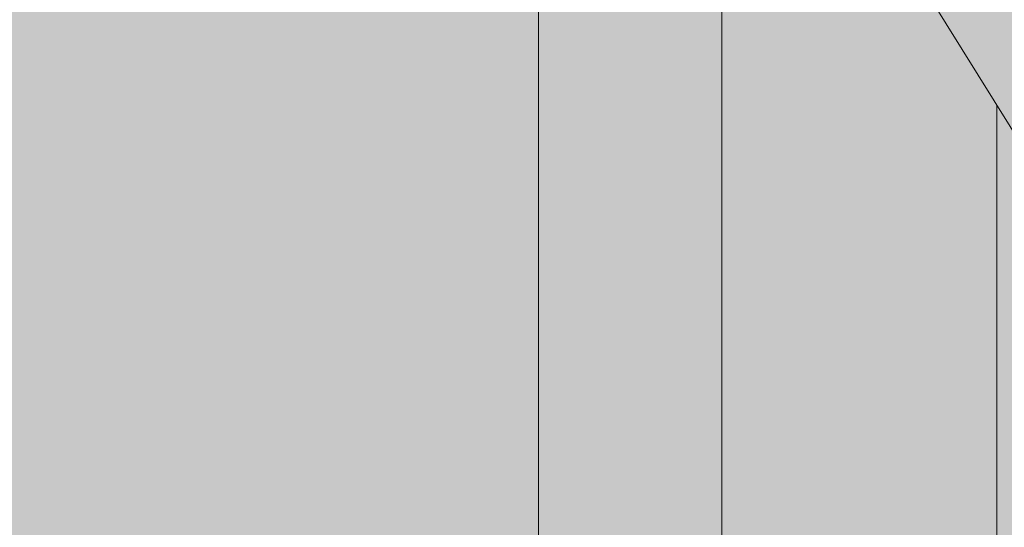
# Model space of a CAD drawing. Units: millimetres. Extents: x 11032 to 26788, y 3406 to 24505.
# Tile 46 of 78: x 15518 to 15786, y 16039 to 16177. Entities that reach past the tile are written whole.
import ezdxf

# ---------------------------------------------------------------- set-up
doc = ezdxf.new("R2010")
doc.units = ezdxf.units.MM
doc.header["$MEASUREMENT"] = 0
for name, color, linetype, lineweight in [('A-ANNO-DIMS', 2, 'Continuous', 18), ('A-GLAZ', 250, 'Continuous', 20), ('A-ROOF', 7, 'Continuous', 30), ('A-WALL', 7, 'Continuous', 35), ('E-LITE', 7, 'Continuous', 18), ('E-LITE-PATT', 7, 'Continuous', 13)]:
    doc.layers.add(name, color=color, linetype=linetype, lineweight=lineweight)
for name, color, linetype, lineweight, true_color in [('A-GLAZ-FRAM-PATT', 250, 'Continuous', 13, 0x262627), ('A-ROOF-PATT', 9, 'Continuous', 13, 0xc7c8ca), ('A-WALL-INTR-PATT', 251, 'Continuous', 13, 0x6c6b6a)]:
    doc.layers.add(name, color=color, linetype=linetype, lineweight=lineweight, true_color=true_color)
doc.styles.get("Standard").update_dxf_attribs({"font": 'arial.ttf'})
doc.dimstyles.get("Standard").update_dxf_attribs({"dimtxt": 150, "dimasz": 100, "dimexe": 10, "dimexo": 5, "dimgap": 5, "dimtad": 0, "dimtih": 1, "dimtoh": 1, "dimdec": 0, "dimzin": 0, "dimdsep": 46, "dimtxsty": 'Standard', "dimcen": 0.09, "dimadec": 0, "dimazin": 0, "dimtfac": 1, "dimtdec": 0, "dimtofl": 0, "dimtmove": 0, "dimatfit": 3, "dimfxl": 1, "dimtolj": 1, "dimtzin": 0, "dimarcsym": 0})

# ---------------------------------------------------------------- blocks, each defined once
blk = doc.blocks.new('*D36')
at = {"layer": 'A-ANNO-DIMS', "color": 0, "lineweight": -2, "transparency": 16777216}
for p, q in [((12301.26, 17115.89), (12301.26, 24416.86)), ((25397.4, 4466.4), (25397.4, 24416.86)), ((12401.26, 24406.86), (18569.2, 24406.86)), ((25297.4, 24406.86), (19129.47, 24406.86))]:
    blk.add_line(p, q, dxfattribs=at)
at = {"layer": 'A-ANNO-DIMS', "color": 0, "transparency": 16777216}
for points in [[(12401.26, 24423.52), (12401.26, 24390.19), (12301.26, 24406.86)], [(25297.4, 24423.52), (25297.4, 24390.19), (25397.4, 24406.86)]]:
    blk.add_solid(points, dxfattribs=at)
at = {"layer": 'Defpoints', "color": 0, "transparency": 16777216}
for p in [(25397.4, 24406.86), (12301.26, 17110.89), (25397.4, 4461.4)]:
    blk.add_point(p, dxfattribs=at)
at = {"layer": 'A-ANNO-DIMS', "color": 0, "transparency": 16777216, "insert": (18849.33, 24406.86), "char_height": 150, "attachment_point": 5}
blk.add_mtext('\\A1;13096', dxfattribs=at)
blk = doc.blocks.new('*D37')
at = {"layer": 'A-ANNO-DIMS', "color": 0, "lineweight": -2, "transparency": 16777216}
for p, q in [((18087.74, 23450.36), (11334.76, 23450.36)), ((11344.76, 23350.36), (11344.76, 14037.46)), ((11344.76, 4561.4), (11344.76, 13874.29)), ((12927.66, 4461.4), (11334.76, 4461.4))]:
    blk.add_line(p, q, dxfattribs=at)
at = {"layer": 'A-ANNO-DIMS', "color": 0, "transparency": 16777216}
for points in [[(11328.1, 23350.36), (11361.43, 23350.36), (11344.76, 23450.36)], [(11328.1, 4561.4), (11361.43, 4561.4), (11344.76, 4461.4)]]:
    blk.add_solid(points, dxfattribs=at)
at = {"layer": 'Defpoints', "color": 0, "transparency": 16777216}
for p in [(11344.76, 23450.36), (18092.74, 23450.36), (12932.66, 4461.4)]:
    blk.add_point(p, dxfattribs=at)
at = {"layer": 'A-ANNO-DIMS', "color": 0, "transparency": 16777216, "insert": (11344.76, 13955.88), "char_height": 150, "attachment_point": 5}
blk.add_mtext('\\A1;18989', dxfattribs=at)
blk = doc.blocks.new('*D57')
at = {"layer": 'A-ANNO-DIMS', "color": 0, "lineweight": -2, "transparency": 16777216}
for p, q in [((14994.7, 7266.4), (14994.7, 24416.86)), ((20894.7, 7266.4), (20894.7, 24416.86)), ((15094.7, 24406.86), (17715.98, 24406.86)), ((20794.7, 24406.86), (18173.42, 24406.86))]:
    blk.add_line(p, q, dxfattribs=at)
at = {"layer": 'A-ANNO-DIMS', "color": 0, "transparency": 16777216}
for points in [[(15094.7, 24423.52), (15094.7, 24390.19), (14994.7, 24406.86)], [(20794.7, 24423.52), (20794.7, 24390.19), (20894.7, 24406.86)]]:
    blk.add_solid(points, dxfattribs=at)
at = {"layer": 'Defpoints', "color": 0, "transparency": 16777216}
for p in [(20894.7, 24406.86), (14994.7, 7261.4), (20894.7, 7261.4)]:
    blk.add_point(p, dxfattribs=at)
at = {"layer": 'A-ANNO-DIMS', "color": 0, "transparency": 16777216, "insert": (17944.7, 24406.86), "char_height": 150, "attachment_point": 5}
blk.add_mtext('\\A1;5900', dxfattribs=at)
blk = doc.blocks.new('*D60')
at = {"layer": 'A-ANNO-DIMS', "color": 0, "lineweight": -2, "transparency": 16777216}
for p, q in [((14994.7, 7266.4), (14994.7, 24416.86)), ((16344.7, 7266.4), (16344.7, 24416.86)), ((15094.7, 24406.86), (15448.04, 24406.86)), ((16244.7, 24406.86), (15891.36, 24406.86))]:
    blk.add_line(p, q, dxfattribs=at)
at = {"layer": 'A-ANNO-DIMS', "color": 0, "transparency": 16777216}
for points in [[(15094.7, 24423.52), (15094.7, 24390.19), (14994.7, 24406.86)], [(16244.7, 24423.52), (16244.7, 24390.19), (16344.7, 24406.86)]]:
    blk.add_solid(points, dxfattribs=at)
at = {"layer": 'Defpoints', "color": 0, "transparency": 16777216}
for p in [(16344.7, 24406.86), (14994.7, 7261.4), (16344.7, 7261.4)]:
    blk.add_point(p, dxfattribs=at)
at = {"layer": 'A-ANNO-DIMS', "color": 0, "transparency": 16777216, "insert": (15669.7, 24406.86), "char_height": 150, "attachment_point": 5}
blk.add_mtext('\\A1;1350', dxfattribs=at)

msp = doc.modelspace()

# ---------------------------------------------------------------- hatches: boundary and pattern name
at = {"layer": 'A-GLAZ-FRAM-PATT'}
h = msp.add_hatch(color=256, dxfattribs=at)
edge = h.paths.add_edge_path()
edge.add_line((15284.393, 17051.32), (15084.393, 17001.32))
edge.add_line((15084.393, 17001.32), (15084.393, 15951.32))
edge.add_spline(control_points=[(15084.393, 15951.32), (15157.266, 15924.219), (15224.458, 15897.808), (15284.393, 15870.289)], knot_values=[511.9490104, 511.9490104, 511.9490104, 511.9490104, 697.3715979, 697.3715979, 697.3715979, 697.3715979], degree=3, periodic=0)
edge.add_line((15284.393, 15870.289), (15284.393, 17051.32))
edge = h.paths.add_edge_path()
edge.add_line((15659.393, 16354.387), (15459.393, 16675.629))
edge.add_line((15459.393, 16675.629), (15459.393, 15771.505))
edge.add_spline(control_points=[(15459.393, 15771.505), (15501.891, 15741.568), (15571.096, 15682.692), (15632.72, 15612.509), (15659.393, 15578.299)], knot_values=[905.064582, 905.064582, 905.064582, 905.064582, 1079.4682707, 1223.1584353, 1223.1584353, 1223.1584353, 1223.1584353], degree=3, periodic=0)
edge.add_line((15659.393, 15578.299), (15659.393, 16354.387))
h.paths.add_polyline_path([(15284.393, 17051.32), (15284.393, 16956.717), (15784.393, 16153.61), (15784.393, 16248.213)])
h = msp.add_hatch(color=256, dxfattribs=at)
edge = h.paths.add_edge_path()
edge.add_spline(control_points=[(15409.393, 16728.446), (15384.197, 16718.122), (15359.177, 16707.259), (15334.393, 16695.842)], knot_values=[2052.6714029, 2052.6714029, 2052.6714029, 2052.6714029, 2131.0201637, 2131.0201637, 2131.0201637, 2131.0201637], degree=3, periodic=0)
edge.add_line((15334.393, 16695.842), (15334.393, 15846.165))
edge.add_spline(control_points=[(15334.393, 15846.165), (15360.99, 15832.635), (15385.89, 15818.741), (15409.393, 15804.345)], knot_values=[750.8383504, 750.8383504, 750.8383504, 750.8383504, 839.4758736, 839.4758736, 839.4758736, 839.4758736], degree=3, periodic=0)
edge.add_line((15409.393, 15804.345), (15409.393, 16728.446))
edge = h.paths.add_edge_path()
edge.add_line((15784.393, 16153.61), (15709.393, 16274.076))
edge.add_line((15709.393, 16274.076), (15709.393, 15509.31))
edge.add_spline(control_points=[(15709.393, 15509.31), (15712.398, 15504.862), (15738.373, 15465.922), (15763.422, 15424.165), (15784.393, 15385.996)], knot_values=[1315.3424293, 1315.3424293, 1315.3424293, 1315.3424293, 1332.3824154, 1463.2850479, 1463.2850479, 1463.2850479, 1463.2850479], degree=3, periodic=0)
edge.add_line((15784.393, 15385.996), (15784.393, 16153.61))
h = msp.add_hatch(color=256, dxfattribs=at)
edge = h.paths.add_edge_path()
edge.add_line((15784.393, 16248.213), (15784.393, 16153.61))
edge.add_line((15784.393, 16153.61), (16560.042, 14907.752))
edge.add_spline(control_points=[(16560.042, 14907.752), (16569.192, 14907.664), (16578.343, 14907.575), (16587.493, 14907.486), (16598.103, 14907.383), (16608.713, 14907.281), (16619.296, 14907.181)], knot_values=[1012.2878735, 1012.2878735, 1012.2878735, 1012.2878735, 1027.155312, 1027.155312, 1027.155312, 1044.3939449, 1044.3939449, 1044.3939449, 1044.3939449], degree=3, periodic=0)
edge.add_line((16619.296, 14907.181), (15784.393, 16248.213))
at = {"layer": 'A-ROOF-PATT'}
h = msp.add_hatch(color=256, dxfattribs=at)
edge = h.paths.add_edge_path()
edge.add_spline(control_points=[(17532.827, 17324.837), (17391.335, 17349.016), (16840.872, 17494.912), (16080.055, 18069.544), (14738.803, 18299.641), (13382.429, 18838.336), (12580.532, 17870.207), (12430.422, 17563.822)], knot_values=[2977.6027945, 2977.6027945, 2977.6027945, 2977.6027945, 3438.1840601, 4811.6463022, 5622.8675483, 7588.0288188, 8560.6685791, 8560.6685791, 8560.6685791, 8560.6685791], degree=3, periodic=0)
edge.add_spline(control_points=[(12430.422, 17563.822), (12437.904, 17573.36), (12445.386, 17582.899), (12452.869, 17592.437), (12452.869, 17592.438), (12452.869, 17592.438), (12452.869, 17592.438)], knot_values=[1408.564138, 1408.564138, 1408.564138, 1408.564138, 1444.85989, 1444.85989, 1444.85989, 1444.8601183, 1444.8601183, 1444.8601183, 1444.8601183], degree=3, periodic=0)
edge.add_spline(control_points=[(12452.869, 17592.438), (12555.432, 17723.185), (12736.557, 17929.686), (13044.86, 18114.643), (13219.943, 18189.644), (13299.92, 18220.646)], knot_values=[339.318246, 339.318246, 339.318246, 339.318246, 836.8349967, 1151.2512933, 1408.564138, 1408.564138, 1408.564138, 1408.564138], degree=3, periodic=0)
edge.add_spline(control_points=[(13299.92, 18220.646), (13299.998, 18220.689), (13300.077, 18220.732), (13319.738, 18231.488), (13339.24, 18241.402), (13388.645, 18264.703), (13418.466, 18277.069), (13478.019, 18298.648), (13507.751, 18307.861), (13544.561, 18317.488), (13551.584, 18319.245), (13558.612, 18320.924)], knot_values=[3783.8950972, 3783.8950972, 3783.8950972, 3783.8950972, 3784.1737101, 3784.1737101, 3853.4666747, 3853.4666747, 3960.2401917, 3960.2401917, 4067.0137087, 4067.0137087, 4092.1744649, 4092.1744649, 4092.1744649, 4092.1744649], degree=3, periodic=0)
edge.add_spline(control_points=[(13558.612, 18320.924), (13581.407, 18326.373), (13604.25, 18331.007), (13657.184, 18339.957), (13687.338, 18343.732), (13748.098, 18348.892), (13778.704, 18350.276), (13840.46, 18350.833), (13871.609, 18350.005), (13934.496, 18346.313), (13966.232, 18343.449), (14030.297, 18335.871), (14062.625, 18331.158), (14127.853, 18320.088), (14160.753, 18313.73), (14241.357, 18296.556), (14289.343, 18284.997), (14386.31, 18259.688), (14435.291, 18245.941), (14534.161, 18217.034), (14584.049, 18201.875), (14684.682, 18170.964), (14735.427, 18155.212), (14837.763, 18123.971), (14889.354, 18108.482), (14954.971, 18089.677), (14968.586, 18085.823), (14992.391, 18079.184), (15002.566, 18076.376), (15021.739, 18071.153), (15030.731, 18068.729), (15047.707, 18064.21), (15055.694, 18062.106), (15079.815, 18055.825), (15095.905, 18051.728), (15143.966, 18039.717), (15175.729, 18032.084), (15254.84, 18013.501), (15301.798, 18002.866), (15394.186, 17981.845), (15439.615, 17971.459), (15528.833, 17950.135), (15572.62, 17939.197), (15658.477, 17916.021), (15700.546, 17903.785), (15753.633, 17886.734), (15765.446, 17882.835), (15786.574, 17875.653), (15795.915, 17872.404), (15810.108, 17867.349), (15814.99, 17865.588), (15824.736, 17862.029), (15829.611, 17860.226), (15844.241, 17854.75), (15854.002, 17851.008), (15883.312, 17839.521), (15902.885, 17831.512), (15966.355, 17804.548), (16010.39, 17784.302), (16098.838, 17741.267), (16143.25, 17718.478), (16232.497, 17671.098), (16277.332, 17646.507), (16367.515, 17596.295), (16412.862, 17570.676), (16504.202, 17519.209), (16550.194, 17493.362), (16643.009, 17442.263), (16689.831, 17417.011), (16756.517, 17382.472), (16775.937, 17372.58), (16795.455, 17362.84)], knot_values=[4092.1744649, 4092.1744649, 4092.1744649, 4092.1744649, 4173.7872258, 4173.7872258, 4280.5607428, 4280.5607428, 4387.3342598, 4387.3342598, 4494.1077768, 4494.1077768, 4600.8812939, 4600.8812939, 4707.6548109, 4707.6548109, 4814.4283279, 4814.4283279, 4967.1262405, 4967.1262405, 5119.8241531, 5119.8241531, 5272.5220657, 5272.5220657, 5425.2199783, 5425.2199783, 5577.9178908, 5577.9178908, 5617.7853319, 5617.7853319, 5647.4648479, 5647.4648479, 5673.611025, 5673.611025, 5696.747607, 5696.747607, 5743.6818903, 5743.6818903, 5837.5504571, 5837.5504571, 5979.7261046, 5979.7261046, 6121.9017521, 6121.9017521, 6264.0773996, 6264.0773996, 6406.2530471, 6406.2530471, 6447.2585849, 6447.2585849, 6480.0420882, 6480.0420882, 6497.3077062, 6497.3077062, 6514.5733242, 6514.5733242, 6549.1045602, 6549.1045602, 6618.1670322, 6618.1670322, 6772.6610171, 6772.6610171, 6927.155002, 6927.155002, 7081.6489869, 7081.6489869, 7236.1429718, 7236.1429718, 7390.6369567, 7390.6369567, 7545.1309416, 7545.1309416, 7608.1992868, 7608.1992868, 7608.1992868, 7608.1992868], degree=3, periodic=0)
edge.add_spline(control_points=[(16795.455, 17362.84), (16814.335, 17349.456), (16832.897, 17336.263), (16873.225, 17307.197), (16894.778, 17291.386), (16936.221, 17259.941), (16956.11, 17244.308), (16993.863, 17213.094), (17011.726, 17197.514), (17041.993, 17169.265), (17054.791, 17156.601), (17078.762, 17131.225), (17089.933, 17118.516), (17110.618, 17092.991), (17120.131, 17080.178), (17130.17, 17065.264), (17131.487, 17063.277), (17133.77, 17059.776), (17134.746, 17058.261), (17136.69, 17055.205), (17137.657, 17053.668), (17140.539, 17049.025), (17142.438, 17045.89), (17148.068, 17036.367), (17151.732, 17029.859), (17163.03, 17008.788), (17170.335, 16993.646), (17184.087, 16961.978), (17190.534, 16945.453), (17202.562, 16911.165), (17208.142, 16893.402), (17218.448, 16856.821), (17223.173, 16838.003), (17231.801, 16799.51), (17235.705, 16779.837), (17241.533, 16746.739), (17243.676, 16733.5), (17247.718, 16706.37), (17249.608, 16692.472), (17252.066, 16672.69), (17252.761, 16666.875), (17254.1, 16655.226), (17254.744, 16649.4), (17256.596, 16631.917), (17257.727, 16620.254), (17260.823, 16585.238), (17262.489, 16561.858), (17266.551, 16488.654), (17267.658, 16438.661), (17267.349, 16375.228), (17267.193, 16362.07), (17266.95, 16348.891)], knot_values=[15.1130472, 15.1130472, 15.1130472, 15.1130472, 82.6995146, 82.6995146, 165.3990291, 165.3990291, 248.0985437, 248.0985437, 330.7980583, 330.7980583, 397.9419458, 397.9419458, 465.0858333, 465.0858333, 532.2297209, 532.2297209, 542.533741, 542.533741, 550.3568158, 550.3568158, 558.1798906, 558.1798906, 573.8260402, 573.8260402, 605.1183395, 605.1183395, 672.7640614, 672.7640614, 740.4097834, 740.4097834, 808.0555054, 808.0555054, 875.7012273, 875.7012273, 943.3469493, 943.3469493, 987.6613492, 987.6613492, 1033.4121612, 1033.4121612, 1052.3850876, 1052.3850876, 1071.358014, 1071.358014, 1109.3038668, 1109.3038668, 1185.1955724, 1185.1955724, 1346.4419026, 1346.4419026, 1388.5586631, 1388.5586631, 1388.5586631, 1388.5586631], degree=3, periodic=0)
edge.add_spline(control_points=[(17266.95, 16348.891), (17266.95, 16348.891), (17266.95, 16348.891), (17266.95, 16348.891), (17253.182, 15602.417), (17239.414, 14855.943), (17225.646, 14109.469)], knot_values=[1388.5586631, 1388.5586631, 1388.5586631, 1388.5586631, 1388.5589654, 1388.5589654, 1388.5589654, 3774.0767661, 3774.0767661, 3774.0767661, 3774.0767661], degree=3, periodic=0)
edge.add_spline(control_points=[(17225.646, 14109.469), (17226.198, 14109.827), (17226.748, 14110.185), (17242.065, 14120.191), (17255.956, 14130.116), (17274.422, 14144.286), (17279.609, 14148.386), (17284.686, 14152.511)], knot_values=[1926.3423968, 1926.3423968, 1926.3423968, 1926.3423968, 1927.316729, 1927.316729, 1953.5121761, 1953.5121761, 1964.0732348, 1964.0732348, 1964.0732348, 1964.0732348], degree=3, periodic=0)
edge.add_spline(control_points=[(17284.686, 14152.511), (17315.791, 14194.761), (17384.413, 14446.273), (17407.128, 14793.401), (17407.093, 15295.84), (17423.274, 15626.362), (17415.601, 15782.507)], knot_values=[0, 0, 0, 0, 163.2554674, 619.2296767, 1171.8624483, 1621.6355562, 1621.6355562, 1621.6355562, 1621.6355562], degree=3, periodic=0)
edge.add_spline(control_points=[(17415.601, 15782.507), (17438.21, 16077.57), (17410.495, 16533.484), (17390.893, 17030.649), (17301.082, 17169.349)], knot_values=[543.9784753, 543.9784753, 543.9784753, 543.9784753, 1452.9852767, 1960.0114926, 1960.0114926, 1960.0114926, 1960.0114926], degree=3, periodic=0)
edge.add_spline(control_points=[(17301.082, 17169.349), (17346.58, 17157.64), (17392.235, 17147.336), (17467.161, 17132.609), (17496.336, 17127.412), (17525.58, 17122.709)], knot_values=[8131.593939, 8131.593939, 8131.593939, 8131.593939, 8269.7349273, 8269.7349273, 8357.5016646, 8357.5016646, 8357.5016646, 8357.5016646], degree=3, periodic=0)
edge.add_line((17525.58, 17122.709), (17532.827, 17324.837))
edge = h.paths.add_edge_path(flags=17)
edge.add_spline(control_points=[(13340.537, 14602.706), (13316.172, 14726.456), (13323.666, 14932.342), (13637.836, 15081.117), (13863.248, 15171.051), (14002.1, 15224.503), (14058.539, 15244.876)], knot_values=[680.8931862, 680.8931862, 680.8931862, 680.8931862, 1033.4728289, 1337.4008326, 1604.7214264, 1784.2944722, 1784.2944722, 1784.2944722, 1784.2944722], degree=3, periodic=0)
edge.add_spline(control_points=[(14058.539, 15244.876), (14058.289, 15275.236), (14057.634, 15305.434), (14055.312, 15376.527), (14053.359, 15417.248), (14048.642, 15497.048), (14045.89, 15536.143), (14042.888, 15574.619)], knot_values=[6573.1065419, 6573.1065419, 6573.1065419, 6573.1065419, 6636.7330012, 6636.7330012, 6723.8890547, 6723.8890547, 6809.6328771, 6809.6328771, 6809.6328771, 6809.6328771], degree=3, periodic=0)
edge.add_spline(control_points=[(14042.888, 15574.619), (13546.54, 15403.221), (13074.735, 15143.241), (13277.36, 14695.339), (13340.537, 14602.706)], knot_values=[503.7925783, 503.7925783, 503.7925783, 503.7925783, 1728.1787606, 2051.34844, 2051.34844, 2051.34844, 2051.34844], degree=3, periodic=0)
h = msp.add_hatch(color=256, dxfattribs=at)
h.set_gradient(color1=(254, 234, 185), color2=(254, 204, 102), name='HEMISPHERICAL')
edge = h.paths.add_edge_path()
edge.add_line((15084.393, 17001.32), (15284.393, 17051.32))
edge.add_line((15284.393, 17051.32), (15470.537, 16752.334))
edge.add_spline(control_points=[(15470.537, 16752.334), (15683.311, 16831.508), (16106.827, 16912.335), (16625.609, 16876.997), (17083.498, 16357.78), (17257.801, 16180.113)], knot_values=[0, 0, 0, 0, 655.2936334, 1252.0157838, 1989.6162859, 1989.6162859, 1989.6162859, 1989.6162859], degree=3, periodic=0)
edge.add_spline(control_points=[(17257.801, 16180.113), (17260.851, 16236.372), (17263.9, 16292.632), (17266.95, 16348.891)], knot_values=[1132.9967717, 1132.9967717, 1132.9967717, 1132.9967717, 1198.0464225, 1198.0464225, 1198.0464225, 1198.0464225], degree=3, periodic=0)
edge.add_spline(control_points=[(17266.95, 16348.891), (17267.193, 16362.07), (17267.349, 16375.228), (17267.658, 16438.661), (17266.551, 16488.654), (17262.489, 16561.858), (17260.823, 16585.238), (17257.727, 16620.254), (17256.596, 16631.917), (17254.744, 16649.4), (17254.1, 16655.226), (17252.761, 16666.875), (17252.066, 16672.69), (17249.608, 16692.472), (17247.718, 16706.37), (17243.676, 16733.5), (17241.533, 16746.739), (17235.705, 16779.837), (17231.801, 16799.51), (17223.173, 16838.003), (17218.448, 16856.821), (17208.142, 16893.402), (17202.562, 16911.165), (17190.534, 16945.453), (17184.087, 16961.978), (17170.335, 16993.646), (17163.03, 17008.788), (17151.732, 17029.859), (17148.068, 17036.367), (17142.438, 17045.89), (17140.539, 17049.025), (17137.657, 17053.668), (17136.69, 17055.205), (17134.746, 17058.261), (17133.77, 17059.776), (17131.487, 17063.277), (17130.17, 17065.264), (17120.131, 17080.178), (17110.618, 17092.991), (17089.933, 17118.516), (17078.762, 17131.225), (17054.791, 17156.601), (17041.993, 17169.265), (17011.726, 17197.514), (16993.863, 17213.094), (16956.11, 17244.308), (16936.221, 17259.941), (16894.778, 17291.386), (16873.225, 17307.197), (16832.897, 17336.263), (16814.335, 17349.456), (16795.455, 17362.84)], knot_values=[15.1130472, 15.1130472, 15.1130472, 15.1130472, 57.2298077, 57.2298077, 218.4761379, 218.4761379, 294.3678435, 294.3678435, 332.3136963, 332.3136963, 351.2866227, 351.2866227, 370.2595491, 370.2595491, 416.0103612, 416.0103612, 460.324761, 460.324761, 527.970483, 527.970483, 595.616205, 595.616205, 663.2619269, 663.2619269, 730.9076489, 730.9076489, 798.5533709, 798.5533709, 829.8456701, 829.8456701, 845.4918197, 845.4918197, 853.3148945, 853.3148945, 861.1379693, 861.1379693, 871.4419895, 871.4419895, 938.585877, 938.585877, 1005.7297645, 1005.7297645, 1072.8736521, 1072.8736521, 1155.5731666, 1155.5731666, 1238.2726812, 1238.2726812, 1320.9721958, 1320.9721958, 1388.5586631, 1388.5586631, 1388.5586631, 1388.5586631], degree=3, periodic=0)
edge.add_spline(control_points=[(16795.455, 17362.84), (16775.937, 17372.58), (16756.517, 17382.472), (16689.831, 17417.011), (16643.009, 17442.263), (16550.194, 17493.362), (16504.202, 17519.209), (16412.862, 17570.676), (16367.515, 17596.295), (16277.332, 17646.507), (16232.497, 17671.098), (16143.25, 17718.478), (16098.838, 17741.267), (16010.39, 17784.302), (15966.355, 17804.548), (15902.885, 17831.512), (15883.312, 17839.521), (15854.002, 17851.008), (15844.241, 17854.75), (15829.611, 17860.226), (15824.736, 17862.029), (15814.99, 17865.588), (15810.108, 17867.349), (15795.915, 17872.404), (15786.574, 17875.653), (15765.446, 17882.835), (15753.633, 17886.734), (15700.546, 17903.785), (15658.477, 17916.021), (15572.62, 17939.197), (15528.833, 17950.135), (15439.615, 17971.459), (15394.186, 17981.845), (15301.798, 18002.866), (15254.84, 18013.501), (15175.729, 18032.084), (15143.966, 18039.717), (15095.905, 18051.728), (15079.815, 18055.825), (15055.694, 18062.106), (15047.707, 18064.21), (15030.731, 18068.729), (15021.739, 18071.153), (15002.566, 18076.376), (14992.391, 18079.184), (14968.586, 18085.823), (14954.971, 18089.677), (14889.354, 18108.482), (14837.763, 18123.971), (14735.427, 18155.212), (14684.682, 18170.964), (14584.049, 18201.875), (14534.161, 18217.034), (14435.291, 18245.941), (14386.31, 18259.688), (14289.343, 18284.997), (14241.357, 18296.556), (14160.753, 18313.73), (14127.853, 18320.088), (14062.625, 18331.158), (14030.297, 18335.871), (13966.232, 18343.449), (13934.496, 18346.313), (13871.609, 18350.005), (13840.46, 18350.833), (13778.704, 18350.276), (13748.098, 18348.892), (13687.338, 18343.732), (13657.184, 18339.957), (13604.25, 18331.007), (13581.407, 18326.373), (13558.612, 18320.924)], knot_values=[4092.1744649, 4092.1744649, 4092.1744649, 4092.1744649, 4155.2428101, 4155.2428101, 4309.736795, 4309.736795, 4464.2307799, 4464.2307799, 4618.7247648, 4618.7247648, 4773.2187497, 4773.2187497, 4927.7127346, 4927.7127346, 5082.2067195, 5082.2067195, 5151.2691915, 5151.2691915, 5185.8004275, 5185.8004275, 5203.0660455, 5203.0660455, 5220.3316635, 5220.3316635, 5253.1151668, 5253.1151668, 5294.1207046, 5294.1207046, 5436.2963521, 5436.2963521, 5578.4719996, 5578.4719996, 5720.6476471, 5720.6476471, 5862.8232946, 5862.8232946, 5956.6918614, 5956.6918614, 6003.6261447, 6003.6261447, 6026.7627267, 6026.7627267, 6052.9089038, 6052.9089038, 6082.5884198, 6082.5884198, 6122.4558609, 6122.4558609, 6275.1537734, 6275.1537734, 6427.851686, 6427.851686, 6580.5495986, 6580.5495986, 6733.2475112, 6733.2475112, 6885.9454238, 6885.9454238, 6992.7189408, 6992.7189408, 7099.4924578, 7099.4924578, 7206.2659749, 7206.2659749, 7313.0394919, 7313.0394919, 7419.8130089, 7419.8130089, 7526.5865259, 7526.5865259, 7608.1992868, 7608.1992868, 7608.1992868, 7608.1992868], degree=3, periodic=0)
edge.add_spline(control_points=[(13558.612, 18320.924), (13472.381, 18287.498), (13386.15, 18254.072), (13299.92, 18220.646), (13299.92, 18220.646), (13299.92, 18220.646), (13299.92, 18220.646)], knot_values=[61.8832457, 61.8832457, 61.8832457, 61.8832457, 339.3179746, 339.3179746, 339.3179746, 339.318246, 339.318246, 339.318246, 339.318246], degree=3, periodic=0)
edge.add_spline(control_points=[(13299.92, 18220.646), (13219.943, 18189.644), (13044.86, 18114.643), (12736.557, 17929.686), (12555.432, 17723.185), (12452.869, 17592.438)], knot_values=[339.318246, 339.318246, 339.318246, 339.318246, 596.6310906, 911.0473872, 1408.564138, 1408.564138, 1408.564138, 1408.564138], degree=3, periodic=0)
edge.add_spline(control_points=[(12452.869, 17592.438), (12452.869, 17592.438), (12452.869, 17592.438), (12452.869, 17592.437), (12445.386, 17582.899), (12437.904, 17573.36), (12430.422, 17563.822)], knot_values=[1408.564138, 1408.564138, 1408.564138, 1408.564138, 1408.5643663, 1408.5643663, 1408.5643663, 1444.8601183, 1444.8601183, 1444.8601183, 1444.8601183], degree=3, periodic=0)
edge.add_spline(control_points=[(12430.422, 17563.822), (12373.797, 17448.248), (12157.302, 16836.764), (12751.985, 16393.69), (13424.325, 15907.903), (14042.888, 15574.619)], knot_values=[0, 0, 0, 0, 366.8993034, 1975.5941082, 2977.6027945, 2977.6027945, 2977.6027945, 2977.6027945], degree=3, periodic=0)
edge.add_spline(control_points=[(14042.888, 15574.619), (14042.839, 15575.252), (14042.789, 15575.886), (14039.681, 15615.607), (14036.366, 15654.052), (14029.551, 15729.305), (14026.05, 15766.114), (14019.175, 15837.686), (14015.8, 15872.45), (13903.823, 16338.596)], knot_values=[6310.2261504, 6310.2261504, 6310.2261504, 6310.2261504, 6311.6383814, 6311.6383814, 6398.7944349, 6398.7944349, 6485.9504884, 6485.9504884, 6573.1065419, 6573.1065419, 6573.1065419, 6573.1065419], degree=3, periodic=0)
edge.add_spline(control_points=[(13903.823, 16338.596), (14237.315, 16236.889), (14456.623, 16167.555), (14614.196, 16115.84)], knot_values=[0, 0, 0, 0, 202.9853419, 202.9853419, 202.9853419, 202.9853419], degree=3, periodic=0)
edge.add_spline(control_points=[(14614.196, 16115.84), (14663.209, 16178.992), (14799.965, 16341.237), (14969.915, 16481.426), (15084.393, 16556.825)], knot_values=[2405.0345045, 2405.0345045, 2405.0345045, 2405.0345045, 2644.8826966, 3039.2707272, 3039.2707272, 3039.2707272, 3039.2707272], degree=3, periodic=0)
edge.add_line((15084.393, 16556.825), (15084.393, 17001.32))
h.paths.add_polyline_path([(14195.599, 17606.181, -1), (14395.599, 17606.181, -1)], flags=16)
h.paths.add_polyline_path([(13310.178, 17032.97, -1), (13510.178, 17032.97, -1)], flags=16)
h = msp.add_hatch(color=256, dxfattribs=at)
h.set_gradient(color1=(254, 234, 185), color2=(254, 204, 102), name='HEMISPHERICAL')
edge = h.paths.add_edge_path()
edge.add_spline(control_points=[(16560.042, 14907.752), (16569.192, 14907.664), (16578.343, 14907.575), (16587.493, 14907.486), (16832.101, 14905.115), (17122.895, 14902.296), (16849.359, 14976.117), (16870.954, 15304.114), (17098.337, 15241.178), (17235.385, 15203.245)], knot_values=[0, 0, 0, 0, 14.8674385, 14.8674385, 14.8674385, 412.2943091, 487.3345915, 708.6416004, 1044.3939449, 1044.3939449, 1044.3939449, 1044.3939449], degree=3, periodic=0)
edge.add_line((16587.504, 14907.486), (16560.207, 14907.486))
edge.add_line((16560.207, 14907.486), (15784.393, 16153.61))
edge.add_line((15784.393, 16153.61), (15784.393, 15385.996))
edge.add_spline(control_points=[(15784.393, 15385.996), (15798.391, 15360.52), (15847.198, 15266.214), (15887.196, 15168.614), (15912.903, 15096.727)], knot_values=[1463.2850479, 1463.2850479, 1463.2850479, 1463.2850479, 1550.659771, 1779.9599361, 1779.9599361, 1779.9599361, 1779.9599361], degree=3, periodic=0)
edge.add_spline(control_points=[(15912.903, 15096.727), (15913.652, 15095.649), (15914.403, 15094.565), (15925.191, 15078.948), (15935.516, 15063.47), (15956.582, 15030.918), (15967.324, 15013.844), (15989.119, 14978.386), (16000.173, 14960.003), (16022.525, 14922.193), (16033.824, 14902.767), (16056.63, 14863.116), (16068.138, 14842.891), (16091.349, 14801.871), (16103.053, 14781.075), (16126.666, 14739.118), (16138.575, 14717.958), (16162.628, 14675.459), (16174.772, 14654.12), (16199.352, 14611.428), (16211.787, 14590.075), (16237.037, 14547.491), (16249.851, 14526.26), (16271.946, 14490.566), (16281.092, 14476.044), (16299.694, 14447.129), (16309.149, 14432.737), (16328.456, 14404.098), (16338.307, 14389.85), (16358.518, 14361.503), (16368.879, 14347.403), (16390.266, 14319.347), (16401.291, 14305.391), (16420.626, 14281.969), (16428.703, 14272.467), (16445.363, 14253.527), (16453.946, 14244.088), (16471.727, 14225.278), (16480.926, 14215.907), (16500.075, 14197.247), (16510.026, 14187.959), (16530.844, 14169.504), (16541.71, 14160.337), (16564.549, 14142.195), (16576.522, 14133.22), (16597.69, 14118.448), (16606.528, 14112.565), (16624.87, 14101.004), (16634.376, 14095.326), (16654.117, 14084.255), (16664.352, 14078.862), (16685.603, 14068.46), (16696.619, 14063.452), (16719.46, 14053.944), (16731.285, 14049.444), (16755.742, 14041.097), (16768.374, 14037.251), (16794.396, 14030.368), (16807.787, 14027.332), (16835.229, 14022.23), (16849.279, 14020.163), (16877.882, 14017.141), (16892.435, 14016.186), (16921.835, 14015.489), (16936.683, 14015.749), (16961.564, 14017.241), (16971.582, 14018.127), (16986.57, 14019.883), (16991.56, 14020.54), (16999.027, 14021.63), (17001.514, 14022.011), (17006.48, 14022.809), (17008.962, 14023.225), (17014.824, 14024.251), (17018.193, 14024.875), (17036.262, 14028.398), (17050.55, 14031.826), (17078.171, 14039.583), (17091.505, 14043.912), (17115.643, 14052.705), (17126.557, 14057.089), (17137.108, 14061.688)], knot_values=[2010.7639617, 2010.7639617, 2010.7639617, 2010.7639617, 2014.7029827, 2014.7029827, 2067.238337, 2067.238337, 2119.7736913, 2119.7736913, 2172.3090457, 2172.3090457, 2224.8444, 2224.8444, 2277.3797543, 2277.3797543, 2329.9151086, 2329.9151086, 2382.450463, 2382.450463, 2434.9858173, 2434.9858173, 2487.5211716, 2487.5211716, 2540.0565259, 2540.0565259, 2576.3179289, 2576.3179289, 2612.5793318, 2612.5793318, 2648.8407347, 2648.8407347, 2685.1021376, 2685.1021376, 2721.3635405, 2721.3635405, 2746.252015, 2746.252015, 2771.1404895, 2771.1404895, 2796.028964, 2796.028964, 2820.9174385, 2820.9174385, 2845.8059131, 2845.8059131, 2870.6943876, 2870.6943876, 2887.5132757, 2887.5132757, 2904.3321639, 2904.3321639, 2921.1510521, 2921.1510521, 2937.9699402, 2937.9699402, 2954.7888284, 2954.7888284, 2971.6077166, 2971.6077166, 2988.4266047, 2988.4266047, 3005.2454929, 3005.2454929, 3022.0643811, 3022.0643811, 3038.8832692, 3038.8832692, 3050.1975453, 3050.1975453, 3055.8546833, 3055.8546833, 3058.6832524, 3058.6832524, 3061.5118214, 3061.5118214, 3065.3934173, 3065.3934173, 3082.4668716, 3082.4668716, 3099.5403259, 3099.5403259, 3114.5433443, 3114.5433443, 3114.5433443, 3114.5433443], degree=3, periodic=0)
edge.add_spline(control_points=[(17137.108, 14061.688), (17165.253, 14274.398), (17209.97, 14653.885), (17230.2, 15035.586), (17235.385, 15203.245)], knot_values=[1968.0804557, 1968.0804557, 1968.0804557, 1968.0804557, 2611.5282875, 3114.5379264, 3114.5379264, 3114.5379264, 3114.5379264], degree=3, periodic=0)
edge = h.paths.add_edge_path()
edge.add_spline(control_points=[(16856.103, 14956.992), (16852.841, 14961.219), (16849.83, 14965.576), (16842.539, 14977.287), (16838.658, 14984.798), (16832.033, 15000.109), (16829.289, 15007.911), (16824.126, 15026.008), (16822.047, 15036.354), (16819.308, 15057.097), (16818.649, 15067.496), (16818.576, 15088.188), (16819.162, 15098.483), (16821.467, 15118.823), (16823.186, 15128.868), (16827.696, 15148.567), (16830.486, 15158.22), (16836.065, 15173.969), (16838.565, 15180.211), (16844.079, 15192.402), (16847.092, 15198.353), (16852.029, 15207.021), (16853.744, 15209.868), (16857.321, 15215.468), (16859.188, 15218.226), (16863.017, 15223.558), (16864.978, 15226.136), (16872.565, 15235.558), (16878.593, 15241.952), (16891.428, 15253.591), (16898.232, 15258.834), (16912.397, 15268.127), (16919.756, 15272.176), (16934.816, 15279.138), (16942.515, 15282.052), (16958.1, 15286.873), (16965.985, 15288.78), (16984.013, 15292.142), (16994.186, 15293.334), (17014.631, 15294.619), (17024.904, 15294.713), (17048.453, 15293.935), (17061.76, 15292.783), (17088.519, 15289.422), (17101.972, 15287.211), (17131.961, 15281.46), (17148.526, 15277.734), (17181.692, 15269.627), (17198.292, 15265.245), (17222.182, 15258.759), (17229.535, 15256.737), (17236.862, 15254.714)], knot_values=[9.6639535, 9.6639535, 9.6639535, 9.6639535, 20.0351668, 20.0351668, 36.9411752, 36.9411752, 53.8471837, 53.8471837, 75.7795687, 75.7795687, 97.7119538, 97.7119538, 119.6443388, 119.6443388, 141.5767238, 141.5767238, 163.5091089, 163.5091089, 178.3829945, 178.3829945, 193.2568801, 193.2568801, 200.6938229, 200.6938229, 208.1307657, 208.1307657, 215.4448585, 215.4448585, 235.5795923, 235.5795923, 255.7143261, 255.7143261, 275.8490598, 275.8490598, 295.9837936, 295.9837936, 316.1185274, 316.1185274, 341.7220543, 341.7220543, 367.3255812, 367.3255812, 400.1572431, 400.1572431, 432.988905, 432.988905, 473.0440165, 473.0440165, 513.099128, 513.099128, 530.9692999, 530.9692999, 530.9692999, 530.9692999], degree=3, periodic=0)
edge.add_spline(control_points=[(17236.862, 15254.714), (17240.377, 15387.456), (17242.496, 15609.536), (17239.752, 15831.567), (17250.544, 16044.717)], knot_values=[1250.9818616, 1250.9818616, 1250.9818616, 1250.9818616, 1649.1516581, 1916.613987, 1916.613987, 1916.613987, 1916.613987], degree=3, periodic=0)
edge.add_spline(control_points=[(17250.544, 16044.717), (17229.169, 16066.505), (17207.794, 16088.292), (17186.419, 16110.08), (17186.418, 16110.08), (17186.418, 16110.081), (17186.418, 16110.081)], knot_values=[-88.5185581, -88.5185581, -88.5185581, -88.5185581, -0.0012784, -0.0012784, -0.0012784, 0, 0, 0, 0], degree=3, periodic=0)
edge.add_spline(control_points=[(17186.418, 16110.081), (17169.261, 16127.569), (17151.499, 16145.947), (17114.892, 16184.084), (17096.046, 16203.842), (17057.437, 16244.305), (17037.673, 16265.01), (16997.415, 16306.918), (16976.921, 16328.12), (16927.79, 16378.347), (16898.924, 16407.388), (16840.771, 16464.327), (16811.484, 16492.225), (16758.449, 16540.764), (16734.666, 16561.798), (16687.634, 16601.588), (16664.382, 16620.344), (16624.116, 16650.909), (16606.897, 16663.324), (16583.769, 16678.999), (16577.49, 16683.149), (16567.144, 16689.805), (16563.039, 16692.397), (16550.823, 16699.959), (16542.775, 16704.739), (16526.841, 16713.814), (16518.956, 16718.108), (16495.524, 16730.301), (16480.199, 16737.514), (16449.97, 16750.334), (16435.066, 16755.942), (16405.476, 16765.764), (16390.79, 16769.979), (16361.418, 16777.195), (16346.731, 16780.197), (16317.147, 16785.133), (16302.249, 16787.067), (16272.053, 16789.992), (16256.756, 16790.981), (16225.609, 16792.125), (16209.759, 16792.279), (16177.385, 16791.865), (16160.862, 16791.296), (16136.98, 16790.07), (16129.942, 16789.661), (16118.22, 16788.91), (16113.574, 16788.594), (16103.645, 16787.886), (16098.362, 16787.489), (16087.761, 16786.652), (16082.439, 16786.212), (16066.413, 16784.825), (16055.649, 16783.812), (16023.135, 16780.505), (16001.164, 16777.942), (15934.539, 16769.141), (15889.17, 16761.791), (15797.417, 16743.949), (15751.033, 16733.457), (15645.217, 16705.796), (15585.74, 16687.58), (15526.207, 16666.217), (15525.367, 16665.915), (15524.528, 16665.613)], knot_values=[0, 0, 0, 0, 71.0501454, 71.0501454, 142.1002909, 142.1002909, 213.1504363, 213.1504363, 284.2005818, 284.2005818, 381.323193, 381.323193, 478.4458043, 478.4458043, 557.8219847, 557.8219847, 637.1981651, 637.1981651, 698.3122593, 698.3122593, 721.3971375, 721.3971375, 736.7790891, 736.7790891, 767.5429924, 767.5429924, 798.3068957, 798.3068957, 859.8347022, 859.8347022, 921.3625088, 921.3625088, 982.8903154, 982.8903154, 1044.4181219, 1044.4181219, 1105.9459285, 1105.9459285, 1167.4737351, 1167.4737351, 1229.0015416, 1229.0015416, 1290.5293482, 1290.5293482, 1315.8990035, 1315.8990035, 1332.3812792, 1332.3812792, 1350.9052657, 1350.9052657, 1369.4292522, 1369.4292522, 1406.4772252, 1406.4772252, 1480.5731712, 1480.5731712, 1628.7650633, 1628.7650633, 1776.9569554, 1776.9569554, 1966.3109251, 1966.3109251, 1969.019495, 1969.019495, 1969.019495, 1969.019495], degree=3, periodic=0)
edge.add_line((15524.528, 16665.613), (16587.978, 14957.484))
edge.add_spline(control_points=[(16587.978, 14957.484), (16605.253, 14957.316), (16622.516, 14957.149), (16665.945, 14956.759), (16691.933, 14956.554), (16742.419, 14956.302), (16766.918, 14956.255), (16813.531, 14956.412), (16835.647, 14956.617), (16856.103, 14956.992)], knot_values=[872.2181925, 872.2181925, 872.2181925, 872.2181925, 900.2857301, 900.2857301, 943.3659889, 943.3659889, 986.4462476, 986.4462476, 1029.5265064, 1029.5265064, 1029.5265064, 1029.5265064], degree=3, periodic=0)
h.paths.add_polyline_path([(16474.605, 15622.642, -1), (16624.605, 15622.642, -1)], flags=16)
h.paths.add_polyline_path([(16198.536, 16037.613, -1), (16348.536, 16037.613, -1)], flags=16)
h.paths.add_polyline_path([(16475.717, 16408.125, -1), (16625.717, 16408.125, -1)], flags=16)
at = {"layer": 'A-WALL-INTR-PATT'}
h = msp.add_hatch(color=256, dxfattribs=at)
edge = h.paths.add_edge_path()
edge.add_line((15334.393, 16876.406), (15284.393, 16956.717))
edge.add_line((15284.393, 16956.717), (15284.393, 15870.289))
edge.add_spline(control_points=[(15284.393, 15870.289), (15297.64, 15864.208), (15314.459, 15856.202), (15330.647, 15848.071), (15334.393, 15846.165)], knot_values=[697.3715979, 697.3715979, 697.3715979, 697.3715979, 738.3518582, 750.8383504, 750.8383504, 750.8383504, 750.8383504], degree=3, periodic=0)
edge.add_line((15334.393, 15846.165), (15334.393, 16876.406))
edge = h.paths.add_edge_path()
edge.add_line((15459.393, 16675.629), (15423.061, 16733.987))
edge.add_spline(control_points=[(15423.061, 16733.987), (15418.499, 16732.158), (15413.944, 16730.311), (15409.393, 16728.446)], knot_values=[2038.5222542, 2038.5222542, 2038.5222542, 2038.5222542, 2052.6714029, 2052.6714029, 2052.6714029, 2052.6714029], degree=3, periodic=0)
edge.add_line((15409.393, 16728.446), (15409.393, 15804.345))
edge.add_spline(control_points=[(15409.393, 15804.345), (15426.785, 15793.692), (15443.411, 15782.764), (15459.393, 15771.505)], knot_values=[839.4758736, 839.4758736, 839.4758736, 839.4758736, 905.064582, 905.064582, 905.064582, 905.064582], degree=3, periodic=0)
edge.add_line((15459.393, 15771.505), (15459.393, 16675.629))
edge = h.paths.add_edge_path()
edge.add_line((15709.393, 16274.076), (15659.393, 16354.387))
edge.add_line((15659.393, 16354.387), (15659.393, 15578.299))
edge.add_spline(control_points=[(15659.393, 15578.299), (15676.505, 15556.352), (15693.138, 15533.373), (15709.393, 15509.31)], knot_values=[1223.1584353, 1223.1584353, 1223.1584353, 1223.1584353, 1315.3424293, 1315.3424293, 1315.3424293, 1315.3424293], degree=3, periodic=0)
edge.add_line((15709.393, 15509.31), (15709.393, 16274.076))
at = {"layer": 'E-LITE-PATT'}
h = msp.add_hatch(color=256, dxfattribs=at)
edge = h.paths.add_edge_path()
edge.add_spline(control_points=[(15084.393, 16556.825), (14969.915, 16481.426), (14799.965, 16341.237), (14663.209, 16178.992), (14614.196, 16115.84)], knot_values=[2405.0345045, 2405.0345045, 2405.0345045, 2405.0345045, 2799.422535, 3039.2707272, 3039.2707272, 3039.2707272, 3039.2707272], degree=3, periodic=0)
edge.add_spline(control_points=[(14614.196, 16115.84), (14650.957, 16103.776), (14684.357, 16092.67), (14715.064, 16082.336)], knot_values=[202.9853419, 202.9853419, 202.9853419, 202.9853419, 250.3408615, 250.3408615, 250.3408615, 250.3408615], degree=3, periodic=0)
edge.add_spline(control_points=[(14715.064, 16082.336), (14732.32, 16103.979), (14749.873, 16125.274), (14780.086, 16160.475), (14792.544, 16174.592), (14817.876, 16202.424), (14830.748, 16216.137), (14853.903, 16239.975), (14864.109, 16250.213), (14884.415, 16270.066), (14894.503, 16279.688), (14918.667, 16302.183), (14932.865, 16314.967), (14987.375, 16362.454), (15029.339, 16395.81), (15076.718, 16430.13), (15080.55, 16432.882), (15084.393, 16435.621)], knot_values=[2472.5855096, 2472.5855096, 2472.5855096, 2472.5855096, 2558.786533, 2558.786533, 2617.7975153, 2617.7975153, 2676.8084975, 2676.8084975, 2721.9976237, 2721.9976237, 2765.3424393, 2765.3424393, 2824.4059302, 2824.4059302, 2988.2351723, 2988.2351723, 3002.5987883, 3002.5987883, 3002.5987883, 3002.5987883], degree=3, periodic=0)
edge.add_line((15084.393, 16435.621), (15084.393, 16556.825))
edge = h.paths.add_edge_path()
edge.add_spline(control_points=[(17257.801, 16180.113), (17083.498, 16357.78), (16625.609, 16876.997), (16106.827, 16912.335), (15683.311, 16831.508), (15470.537, 16752.334)], knot_values=[0, 0, 0, 0, 737.600502, 1334.3226525, 1989.6162859, 1989.6162859, 1989.6162859, 1989.6162859], degree=3, periodic=0)
edge.add_line((15470.537, 16752.334), (15524.528, 16665.613))
edge.add_spline(control_points=[(15524.528, 16665.613), (15525.367, 16665.915), (15526.207, 16666.217), (15585.74, 16687.58), (15645.217, 16705.796), (15751.033, 16733.457), (15797.417, 16743.949), (15889.17, 16761.791), (15934.539, 16769.141), (16001.164, 16777.942), (16023.135, 16780.505), (16055.649, 16783.812), (16066.413, 16784.825), (16082.439, 16786.212), (16087.761, 16786.652), (16098.362, 16787.489), (16103.645, 16787.886), (16113.574, 16788.594), (16118.22, 16788.91), (16129.942, 16789.661), (16136.98, 16790.07), (16160.862, 16791.296), (16177.385, 16791.865), (16209.759, 16792.279), (16225.609, 16792.125), (16256.756, 16790.981), (16272.053, 16789.992), (16302.249, 16787.067), (16317.147, 16785.133), (16346.731, 16780.197), (16361.418, 16777.195), (16390.79, 16769.979), (16405.476, 16765.764), (16435.066, 16755.942), (16449.97, 16750.334), (16480.199, 16737.514), (16495.524, 16730.301), (16518.956, 16718.108), (16526.841, 16713.814), (16542.775, 16704.739), (16550.823, 16699.959), (16563.039, 16692.397), (16567.144, 16689.805), (16577.49, 16683.149), (16583.769, 16678.999), (16606.897, 16663.324), (16624.116, 16650.909), (16664.382, 16620.344), (16687.634, 16601.588), (16734.666, 16561.798), (16758.449, 16540.764), (16811.484, 16492.225), (16840.771, 16464.327), (16898.924, 16407.388), (16927.79, 16378.347), (16976.921, 16328.12), (16997.415, 16306.918), (17037.673, 16265.01), (17057.437, 16244.305), (17096.046, 16203.842), (17114.892, 16184.084), (17151.499, 16145.947), (17169.261, 16127.569), (17186.418, 16110.081)], knot_values=[0, 0, 0, 0, 2.7085699, 2.7085699, 192.0625397, 192.0625397, 340.2544317, 340.2544317, 488.4463238, 488.4463238, 562.5422698, 562.5422698, 599.5902428, 599.5902428, 618.1142294, 618.1142294, 636.6382159, 636.6382159, 653.1204915, 653.1204915, 678.4901469, 678.4901469, 740.0179534, 740.0179534, 801.54576, 801.54576, 863.0735665, 863.0735665, 924.6013731, 924.6013731, 986.1291797, 986.1291797, 1047.6569862, 1047.6569862, 1109.1847928, 1109.1847928, 1170.7125993, 1170.7125993, 1201.4765026, 1201.4765026, 1232.2404059, 1232.2404059, 1247.6223576, 1247.6223576, 1270.7072358, 1270.7072358, 1331.8213299, 1331.8213299, 1411.1975103, 1411.1975103, 1490.5736908, 1490.5736908, 1587.696302, 1587.696302, 1684.8189133, 1684.8189133, 1755.8690587, 1755.8690587, 1826.9192041, 1826.9192041, 1897.9693496, 1897.9693496, 1969.019495, 1969.019495, 1969.019495, 1969.019495], degree=3, periodic=0)
edge.add_spline(control_points=[(17186.418, 16110.081), (17186.418, 16110.081), (17186.418, 16110.08), (17186.419, 16110.08), (17207.794, 16088.292), (17229.169, 16066.505), (17250.544, 16044.717)], knot_values=[-88.5185581, -88.5185581, -88.5185581, -88.5185581, -88.5172797, -88.5172797, -88.5172797, 0, 0, 0, 0], degree=3, periodic=0)
edge.add_spline(control_points=[(17250.544, 16044.717), (17251.307, 16059.803), (17252.131, 16075.51), (17253.018, 16091.882)], knot_values=[1232.05171, 1232.05171, 1232.05171, 1232.05171, 1250.9818616, 1250.9818616, 1250.9818616, 1250.9818616], degree=3, periodic=0)
edge.add_spline(control_points=[(17253.018, 16091.882), (17253.019, 16091.892), (17253.019, 16091.901), (17253.02, 16091.911), (17254.614, 16121.312), (17256.207, 16150.712), (17257.801, 16180.113)], knot_values=[1198.0464225, 1198.0464225, 1198.0464225, 1198.0464225, 1198.0576047, 1198.0576047, 1198.0576047, 1232.05171, 1232.05171, 1232.05171, 1232.05171], degree=3, periodic=0)

# ---------------------------------------------------------------- linework, layer by layer
at = {"layer": 'A-GLAZ'}
for p, q in [((15284.393, 16956.717), (16560.207, 14907.486)), ((15659.393, 15578.299), (15659.393, 16354.387)), ((15709.393, 15509.31), (15709.393, 16274.076)), ((15784.393, 15385.996), (15784.393, 16153.61))]:
    msp.add_line(p, q, dxfattribs=at)
at = {"layer": 'A-ROOF'}
msp.add_open_spline([(14042.888, 15574.619), (13424.325, 15907.903), (12751.985, 16393.69), (11963.048, 16981.495), (13249.687, 18891.056), (14738.803, 18299.641), (16080.055, 18069.544), (16966.203, 17400.251), (17654.208, 17293.942), (17944.704, 17286.735)], degree=3, knots=[0, 0, 0, 0, 1002.0086862, 2610.7034911, 3950.2425548, 5915.4038253, 6726.6250714, 8100.0873135, 8996.4318779, 8996.4318779, 8996.4318779, 8996.4318779], dxfattribs=at)
at = {"layer": 'A-WALL'}
msp.add_open_spline([(13903.823, 16338.596), (14592.588, 16128.54), (14947.845, 16001.782), (15353.854, 15853.294), (15563.925, 15701.294), (15714.647, 15512.154), (15830.664, 15306.558), (15887.196, 15168.614), (15912.903, 15096.727)], degree=3, knots=[0, 0, 0, 0, 419.2278857, 738.3518582, 1079.4682707, 1332.3824154, 1550.659771, 1779.9599361, 1779.9599361, 1779.9599361, 1779.9599361], dxfattribs=at)
at = {"layer": 'E-LITE'}
msp.add_open_spline([(17250.544, 16044.717), (17229.169, 16066.505), (17207.794, 16088.292), (17186.419, 16110.08), (17186.418, 16110.08), (17186.418, 16110.081), (17186.418, 16110.081), (17169.261, 16127.569), (17151.499, 16145.947), (17114.892, 16184.084), (17096.046, 16203.842), (17057.437, 16244.305), (17037.673, 16265.01), (16997.415, 16306.918), (16976.921, 16328.12), (16927.79, 16378.347), (16898.924, 16407.388), (16840.771, 16464.327), (16811.484, 16492.225), (16758.449, 16540.764), (16734.666, 16561.798), (16687.634, 16601.588), (16664.382, 16620.344), (16624.116, 16650.909), (16606.897, 16663.324), (16583.769, 16678.999), (16577.49, 16683.149), (16567.144, 16689.805), (16563.039, 16692.397), (16550.823, 16699.959), (16542.775, 16704.739), (16526.841, 16713.814), (16518.956, 16718.108), (16495.524, 16730.301), (16480.199, 16737.514), (16449.97, 16750.334), (16435.066, 16755.942), (16405.476, 16765.764), (16390.79, 16769.979), (16361.418, 16777.195), (16346.731, 16780.197), (16317.147, 16785.133), (16302.249, 16787.067), (16272.053, 16789.992), (16256.756, 16790.981), (16225.609, 16792.125), (16209.759, 16792.279), (16177.385, 16791.865), (16160.862, 16791.296), (16136.98, 16790.07), (16129.942, 16789.661), (16118.22, 16788.91), (16113.574, 16788.594), (16103.645, 16787.886), (16098.362, 16787.489), (16087.761, 16786.652), (16082.439, 16786.212), (16066.413, 16784.825), (16055.649, 16783.812), (16023.135, 16780.505), (16001.164, 16777.942), (15934.539, 16769.141), (15889.17, 16761.791), (15797.417, 16743.949), (15751.033, 16733.457), (15645.217, 16705.796), (15585.74, 16687.58), (15526.207, 16666.217), (15525.367, 16665.915), (15524.528, 16665.613)], degree=3, knots=[-88.5185581, -88.5185581, -88.5185581, -88.5185581, -0.0012784, -0.0012784, -0.0012784, 0, 0, 0, 71.0501454, 71.0501454, 142.1002909, 142.1002909, 213.1504363, 213.1504363, 284.2005818, 284.2005818, 381.323193, 381.323193, 478.4458043, 478.4458043, 557.8219847, 557.8219847, 637.1981651, 637.1981651, 698.3122593, 698.3122593, 721.3971375, 721.3971375, 736.7790891, 736.7790891, 767.5429924, 767.5429924, 798.3068957, 798.3068957, 859.8347022, 859.8347022, 921.3625088, 921.3625088, 982.8903154, 982.8903154, 1044.4181219, 1044.4181219, 1105.9459285, 1105.9459285, 1167.4737351, 1167.4737351, 1229.0015416, 1229.0015416, 1290.5293482, 1290.5293482, 1315.8990035, 1315.8990035, 1332.3812792, 1332.3812792, 1350.9052657, 1350.9052657, 1369.4292522, 1369.4292522, 1406.4772252, 1406.4772252, 1480.5731712, 1480.5731712, 1628.7650633, 1628.7650633, 1776.9569554, 1776.9569554, 1966.3109251, 1966.3109251, 1969.019495, 1969.019495, 1969.019495, 1969.019495], dxfattribs=at)

# ---------------------------------------------------------------- dimensions: what is measured, and where the dimension line sits
at = {"layer": 'A-ANNO-DIMS'}
for base, p1, p2, picture, middle in [((25397.404, 24406.858), (12301.265, 17110.885), (25397.404, 4461.399), '*D36', (18849.334, 24406.858)), ((20894.704, 24406.858), (14994.704, 7261.399), (20894.704, 7261.399), '*D57', (17944.704, 24406.858)), ((16344.704, 24406.858), (14994.704, 7261.399), (16344.704, 7261.399), '*D60', (15669.704, 24406.858))]:
    dim = msp.add_linear_dim(base=base, p1=p1, p2=p2, dimstyle='Standard', override={"dimdec": 0, "dimlfac": 1, "dimrnd": 0, "dimzin": 0, "dimdsep": 46, "dimlunit": 2}, dxfattribs=at)
    dim.commit()
    dim.dimension.update_dxf_attribs({"geometry": picture, "text_midpoint": middle})
dim = msp.add_linear_dim(base=(11344.765, 23450.358), p1=(12932.665, 4461.399), p2=(18092.739, 23450.358), angle=90, dimstyle='Standard', override={"dimdec": 0, "dimlfac": 1, "dimrnd": 0, "dimzin": 0, "dimdsep": 46, "dimlunit": 2}, dxfattribs=at)
dim.commit()
dim.dimension.update_dxf_attribs({"geometry": '*D37', "text_midpoint": (11344.765, 13955.879)})

doc.saveas('drawing.dxf')
